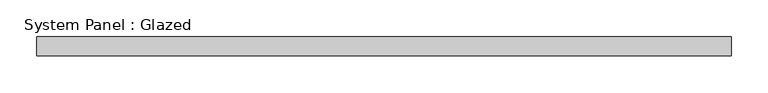
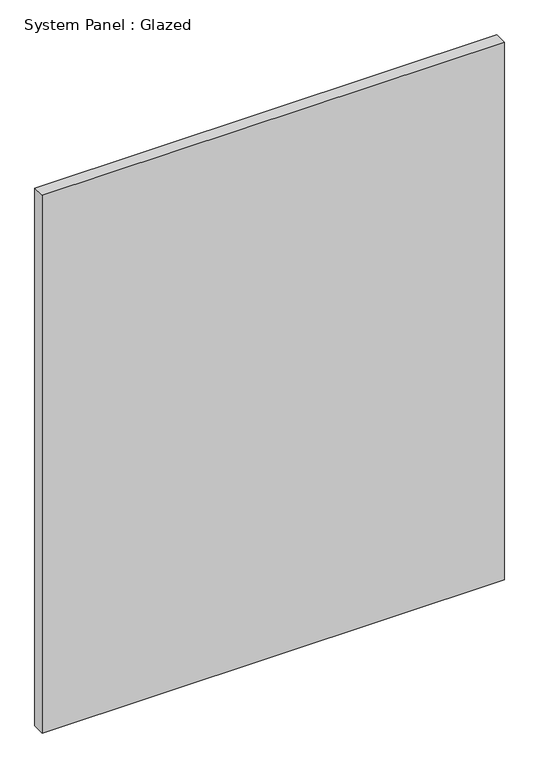
"""IFC4 building model written with IfcOpenShell, lengths in millimetres: plate geometry, System Panel : Glazed."""

from ifc_helpers import new_model, si_unit, origin, origin_with_axes, place, context, project, spatial, polyline, outline, extrude, source, transform, mapped, element, save


def system_panel_glazed_f6e6087a(model_context):
    return source(origin(), model_context, "Body", "SweptSolid", [
        extrude(outline(polyline([(469.9, 19.05), (-469.9, 19.05), (-469.9, 44.45), (469.9, 44.45), (469.9, 19.05)])), origin_with_axes(), (0.0, 0.0, 1.0), 1155.7),
    ])


if __name__ == "__main__":
    model = new_model("IFC4")
    model_context = context("Model", 3, world=origin())
    ifc_project = project(units=[si_unit("LENGTHUNIT", "METRE", prefix="MILLI")], contexts=[model_context])
    site = spatial("IfcSite", under=ifc_project)
    building = spatial("IfcBuilding", under=site)
    placement = place(None, origin())
    system_panel_glazed_shape = system_panel_glazed_f6e6087a(model_context)
    element("IfcPlate", 1, ObjectType="System Panel : Glazed", at=placement, inside=building, context=model_context, shape_type="MappedRepresentation", body=[
        mapped(system_panel_glazed_shape, transform((0.0, 0.0, 0.0), x_axis=(1.0, 0.0, 0.0), y_axis=(0.0, 1.0, 0.0), z_axis=(0.0, 0.0, 1.0))),
    ])
    save(model, "model.ifc")

# Revit data of these elements
# Type "System Panel : Glazed"
#   Construction Type Id = "GSP4R"
#   Analytic Construction = "1/8 in Pilkington single glazing"
#   Visual Light Transmittance = 0.9
#   Solar Heat Gain Coefficient = 0.86
#   Heat Transfer Coefficient (U) = 1.18115 BTU/(h·ft²·°F)
#   Define Thermal Properties by = 1
# Element 1 (IfcPlate, "System Panel : Glazed")
#   Materials on its faces: "Glass"
# Materials
#   "Glass": class "Glass", colour RGB 0 128 192, transparency 0.75, Description = "Soda Lime Glass", Cost = 0
